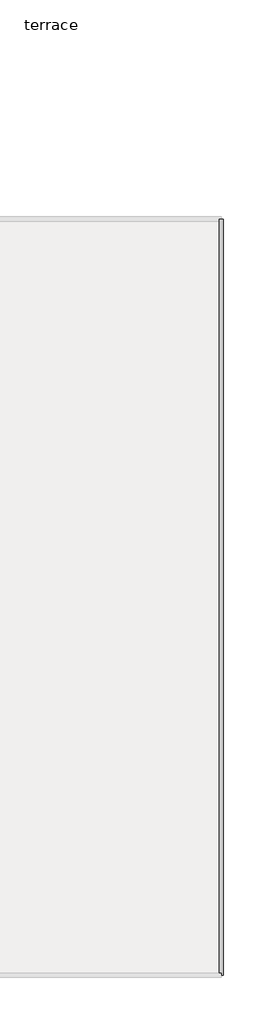
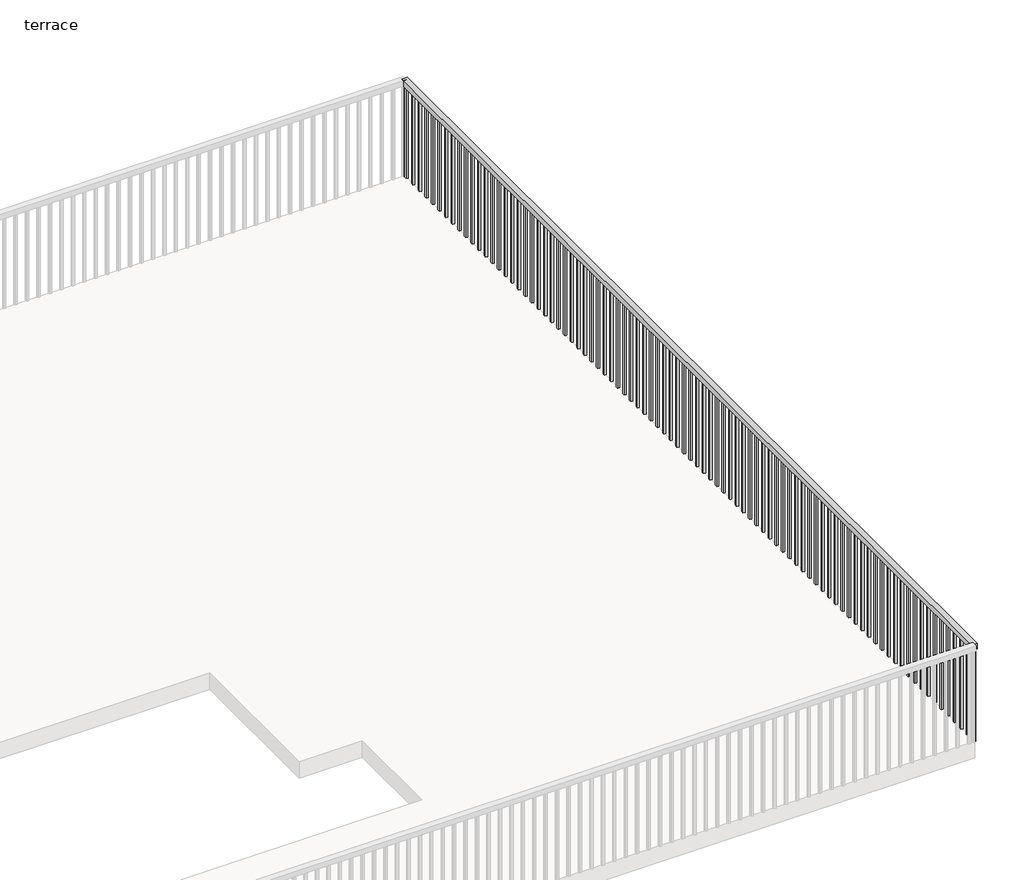
# One storey, part 3 of 4: 1 railing.
"""IFC4 building model written with IfcOpenShell, lengths in millimetres."""

from ifc_helpers import new_model, si_unit, frame, origin, place, context, project, spatial, polyline, outline, extrude, element, save

model = new_model("IFC4")

# Units and contexts
model_context = context("Model", 3, world=origin())
ifc_project = project(units=[si_unit("LENGTHUNIT", "METRE", prefix="MILLI")], contexts=[model_context])

# Site, building, storey
site = spatial("IfcSite", under=ifc_project)
building = spatial("IfcBuilding", under=site)
storey = spatial("IfcBuildingStorey", under=building, Name="terrace", Elevation=7010.4)

# Railing
placement = place(None, origin())
element("IfcRailing", 1, ObjectType="Handrail - Rectangular", at=placement, inside=storey, context=model_context, shape_type="SweptSolid", body=[
    extrude(outline(polyline([(36180.1316163, 5593.0480552), (36129.3316163, 5593.0480552), (36129.3316163, 14362.3980552), (36180.1316163, 14362.3980552), (36180.1316163, 5593.0480552)])), frame((0.0, 0.0, 7874.0), z_axis=(0.0, 0.0, 1.0), x_axis=(1.0, 0.0, 0.0)), (0.0, 0.0, 1.0), 50.8),
    extrude(outline(polyline([(36164.2566163, 14321.1230552), (36145.2066163, 14321.1230552), (36145.2066163, 14340.1730552), (36164.2566163, 14340.1730552), (36164.2566163, 14321.1230552)])), frame((0.0, 0.0, 7010.4), z_axis=(0.0, 0.0, 1.0), x_axis=(1.0, 0.0, 0.0)), (0.0, 0.0, 1.0), 863.6),
    extrude(outline(polyline([(36164.2566163, 14219.5230552), (36145.2066163, 14219.5230552), (36145.2066163, 14238.5730552), (36164.2566163, 14238.5730552), (36164.2566163, 14219.5230552)])), frame((0.0, 0.0, 7010.4), z_axis=(0.0, 0.0, 1.0), x_axis=(1.0, 0.0, 0.0)), (0.0, 0.0, 1.0), 863.6),
    extrude(outline(polyline([(36164.2566163, 14117.9230552), (36145.2066163, 14117.9230552), (36145.2066163, 14136.9730552), (36164.2566163, 14136.9730552), (36164.2566163, 14117.9230552)])), frame((0.0, 0.0, 7010.4), z_axis=(0.0, 0.0, 1.0), x_axis=(1.0, 0.0, 0.0)), (0.0, 0.0, 1.0), 863.6),
    extrude(outline(polyline([(36164.2566163, 14016.3230552), (36145.2066163, 14016.3230552), (36145.2066163, 14035.3730552), (36164.2566163, 14035.3730552), (36164.2566163, 14016.3230552)])), frame((0.0, 0.0, 7010.4), z_axis=(0.0, 0.0, 1.0), x_axis=(1.0, 0.0, 0.0)), (0.0, 0.0, 1.0), 863.6),
    extrude(outline(polyline([(36164.2566163, 13914.7230552), (36145.2066163, 13914.7230552), (36145.2066163, 13933.7730552), (36164.2566163, 13933.7730552), (36164.2566163, 13914.7230552)])), frame((0.0, 0.0, 7010.4), z_axis=(0.0, 0.0, 1.0), x_axis=(1.0, 0.0, 0.0)), (0.0, 0.0, 1.0), 863.6),
    extrude(outline(polyline([(36164.2566163, 13813.1230552), (36145.2066163, 13813.1230552), (36145.2066163, 13832.1730552), (36164.2566163, 13832.1730552), (36164.2566163, 13813.1230552)])), frame((0.0, 0.0, 7010.4), z_axis=(0.0, 0.0, 1.0), x_axis=(1.0, 0.0, 0.0)), (0.0, 0.0, 1.0), 863.6),
    extrude(outline(polyline([(36164.2566163, 13711.5230552), (36145.2066163, 13711.5230552), (36145.2066163, 13730.5730552), (36164.2566163, 13730.5730552), (36164.2566163, 13711.5230552)])), frame((0.0, 0.0, 7010.4), z_axis=(0.0, 0.0, 1.0), x_axis=(1.0, 0.0, 0.0)), (0.0, 0.0, 1.0), 863.6),
    extrude(outline(polyline([(36164.2566163, 13609.9230552), (36145.2066163, 13609.9230552), (36145.2066163, 13628.9730552), (36164.2566163, 13628.9730552), (36164.2566163, 13609.9230552)])), frame((0.0, 0.0, 7010.4), z_axis=(0.0, 0.0, 1.0), x_axis=(1.0, 0.0, 0.0)), (0.0, 0.0, 1.0), 863.6),
    extrude(outline(polyline([(36164.2566163, 13508.3230552), (36145.2066163, 13508.3230552), (36145.2066163, 13527.3730552), (36164.2566163, 13527.3730552), (36164.2566163, 13508.3230552)])), frame((0.0, 0.0, 7010.4), z_axis=(0.0, 0.0, 1.0), x_axis=(1.0, 0.0, 0.0)), (0.0, 0.0, 1.0), 863.6),
    extrude(outline(polyline([(36164.2566163, 13406.7230552), (36145.2066163, 13406.7230552), (36145.2066163, 13425.7730552), (36164.2566163, 13425.7730552), (36164.2566163, 13406.7230552)])), frame((0.0, 0.0, 7010.4), z_axis=(0.0, 0.0, 1.0), x_axis=(1.0, 0.0, 0.0)), (0.0, 0.0, 1.0), 863.6),
    extrude(outline(polyline([(36164.2566163, 13305.1230552), (36145.2066163, 13305.1230552), (36145.2066163, 13324.1730552), (36164.2566163, 13324.1730552), (36164.2566163, 13305.1230552)])), frame((0.0, 0.0, 7010.4), z_axis=(0.0, 0.0, 1.0), x_axis=(1.0, 0.0, 0.0)), (0.0, 0.0, 1.0), 863.6),
    extrude(outline(polyline([(36164.2566163, 13203.5230552), (36145.2066163, 13203.5230552), (36145.2066163, 13222.5730552), (36164.2566163, 13222.5730552), (36164.2566163, 13203.5230552)])), frame((0.0, 0.0, 7010.4), z_axis=(0.0, 0.0, 1.0), x_axis=(1.0, 0.0, 0.0)), (0.0, 0.0, 1.0), 863.6),
    extrude(outline(polyline([(36164.2566163, 13101.9230552), (36145.2066163, 13101.9230552), (36145.2066163, 13120.9730552), (36164.2566163, 13120.9730552), (36164.2566163, 13101.9230552)])), frame((0.0, 0.0, 7010.4), z_axis=(0.0, 0.0, 1.0), x_axis=(1.0, 0.0, 0.0)), (0.0, 0.0, 1.0), 863.6),
    extrude(outline(polyline([(36164.2566163, 13000.3230552), (36145.2066163, 13000.3230552), (36145.2066163, 13019.3730552), (36164.2566163, 13019.3730552), (36164.2566163, 13000.3230552)])), frame((0.0, 0.0, 7010.4), z_axis=(0.0, 0.0, 1.0), x_axis=(1.0, 0.0, 0.0)), (0.0, 0.0, 1.0), 863.6),
    extrude(outline(polyline([(36164.2566163, 12898.7230552), (36145.2066163, 12898.7230552), (36145.2066163, 12917.7730552), (36164.2566163, 12917.7730552), (36164.2566163, 12898.7230552)])), frame((0.0, 0.0, 7010.4), z_axis=(0.0, 0.0, 1.0), x_axis=(1.0, 0.0, 0.0)), (0.0, 0.0, 1.0), 863.6),
    extrude(outline(polyline([(36164.2566163, 12797.1230552), (36145.2066163, 12797.1230552), (36145.2066163, 12816.1730552), (36164.2566163, 12816.1730552), (36164.2566163, 12797.1230552)])), frame((0.0, 0.0, 7010.4), z_axis=(0.0, 0.0, 1.0), x_axis=(1.0, 0.0, 0.0)), (0.0, 0.0, 1.0), 863.6),
    extrude(outline(polyline([(36164.2566163, 12695.5230552), (36145.2066163, 12695.5230552), (36145.2066163, 12714.5730552), (36164.2566163, 12714.5730552), (36164.2566163, 12695.5230552)])), frame((0.0, 0.0, 7010.4), z_axis=(0.0, 0.0, 1.0), x_axis=(1.0, 0.0, 0.0)), (0.0, 0.0, 1.0), 863.6),
    extrude(outline(polyline([(36164.2566163, 12593.9230552), (36145.2066163, 12593.9230552), (36145.2066163, 12612.9730552), (36164.2566163, 12612.9730552), (36164.2566163, 12593.9230552)])), frame((0.0, 0.0, 7010.4), z_axis=(0.0, 0.0, 1.0), x_axis=(1.0, 0.0, 0.0)), (0.0, 0.0, 1.0), 863.6),
    extrude(outline(polyline([(36164.2566163, 12492.3230552), (36145.2066163, 12492.3230552), (36145.2066163, 12511.3730552), (36164.2566163, 12511.3730552), (36164.2566163, 12492.3230552)])), frame((0.0, 0.0, 7010.4), z_axis=(0.0, 0.0, 1.0), x_axis=(1.0, 0.0, 0.0)), (0.0, 0.0, 1.0), 863.6),
    extrude(outline(polyline([(36164.2566163, 12390.7230552), (36145.2066163, 12390.7230552), (36145.2066163, 12409.7730552), (36164.2566163, 12409.7730552), (36164.2566163, 12390.7230552)])), frame((0.0, 0.0, 7010.4), z_axis=(0.0, 0.0, 1.0), x_axis=(1.0, 0.0, 0.0)), (0.0, 0.0, 1.0), 863.6),
    extrude(outline(polyline([(36164.2566163, 12289.1230552), (36145.2066163, 12289.1230552), (36145.2066163, 12308.1730552), (36164.2566163, 12308.1730552), (36164.2566163, 12289.1230552)])), frame((0.0, 0.0, 7010.4), z_axis=(0.0, 0.0, 1.0), x_axis=(1.0, 0.0, 0.0)), (0.0, 0.0, 1.0), 863.6),
    extrude(outline(polyline([(36164.2566163, 12187.5230552), (36145.2066163, 12187.5230552), (36145.2066163, 12206.5730552), (36164.2566163, 12206.5730552), (36164.2566163, 12187.5230552)])), frame((0.0, 0.0, 7010.4), z_axis=(0.0, 0.0, 1.0), x_axis=(1.0, 0.0, 0.0)), (0.0, 0.0, 1.0), 863.6),
    extrude(outline(polyline([(36164.2566163, 12085.9230552), (36145.2066163, 12085.9230552), (36145.2066163, 12104.9730552), (36164.2566163, 12104.9730552), (36164.2566163, 12085.9230552)])), frame((0.0, 0.0, 7010.4), z_axis=(0.0, 0.0, 1.0), x_axis=(1.0, 0.0, 0.0)), (0.0, 0.0, 1.0), 863.6),
    extrude(outline(polyline([(36164.2566163, 11984.3230552), (36145.2066163, 11984.3230552), (36145.2066163, 12003.3730552), (36164.2566163, 12003.3730552), (36164.2566163, 11984.3230552)])), frame((0.0, 0.0, 7010.4), z_axis=(0.0, 0.0, 1.0), x_axis=(1.0, 0.0, 0.0)), (0.0, 0.0, 1.0), 863.6),
    extrude(outline(polyline([(36164.2566163, 11882.7230552), (36145.2066163, 11882.7230552), (36145.2066163, 11901.7730552), (36164.2566163, 11901.7730552), (36164.2566163, 11882.7230552)])), frame((0.0, 0.0, 7010.4), z_axis=(0.0, 0.0, 1.0), x_axis=(1.0, 0.0, 0.0)), (0.0, 0.0, 1.0), 863.6),
    extrude(outline(polyline([(36164.2566163, 11781.1230552), (36145.2066163, 11781.1230552), (36145.2066163, 11800.1730552), (36164.2566163, 11800.1730552), (36164.2566163, 11781.1230552)])), frame((0.0, 0.0, 7010.4), z_axis=(0.0, 0.0, 1.0), x_axis=(1.0, 0.0, 0.0)), (0.0, 0.0, 1.0), 863.6),
    extrude(outline(polyline([(36164.2566163, 11679.5230552), (36145.2066163, 11679.5230552), (36145.2066163, 11698.5730552), (36164.2566163, 11698.5730552), (36164.2566163, 11679.5230552)])), frame((0.0, 0.0, 7010.4), z_axis=(0.0, 0.0, 1.0), x_axis=(1.0, 0.0, 0.0)), (0.0, 0.0, 1.0), 863.6),
    extrude(outline(polyline([(36164.2566163, 11577.9230552), (36145.2066163, 11577.9230552), (36145.2066163, 11596.9730552), (36164.2566163, 11596.9730552), (36164.2566163, 11577.9230552)])), frame((0.0, 0.0, 7010.4), z_axis=(0.0, 0.0, 1.0), x_axis=(1.0, 0.0, 0.0)), (0.0, 0.0, 1.0), 863.6),
    extrude(outline(polyline([(36164.2566163, 11476.3230552), (36145.2066163, 11476.3230552), (36145.2066163, 11495.3730552), (36164.2566163, 11495.3730552), (36164.2566163, 11476.3230552)])), frame((0.0, 0.0, 7010.4), z_axis=(0.0, 0.0, 1.0), x_axis=(1.0, 0.0, 0.0)), (0.0, 0.0, 1.0), 863.6),
    extrude(outline(polyline([(36164.2566163, 11374.7230552), (36145.2066163, 11374.7230552), (36145.2066163, 11393.7730552), (36164.2566163, 11393.7730552), (36164.2566163, 11374.7230552)])), frame((0.0, 0.0, 7010.4), z_axis=(0.0, 0.0, 1.0), x_axis=(1.0, 0.0, 0.0)), (0.0, 0.0, 1.0), 863.6),
    extrude(outline(polyline([(36164.2566163, 11273.1230552), (36145.2066163, 11273.1230552), (36145.2066163, 11292.1730552), (36164.2566163, 11292.1730552), (36164.2566163, 11273.1230552)])), frame((0.0, 0.0, 7010.4), z_axis=(0.0, 0.0, 1.0), x_axis=(1.0, 0.0, 0.0)), (0.0, 0.0, 1.0), 863.6),
    extrude(outline(polyline([(36164.2566163, 11171.5230552), (36145.2066163, 11171.5230552), (36145.2066163, 11190.5730552), (36164.2566163, 11190.5730552), (36164.2566163, 11171.5230552)])), frame((0.0, 0.0, 7010.4), z_axis=(0.0, 0.0, 1.0), x_axis=(1.0, 0.0, 0.0)), (0.0, 0.0, 1.0), 863.6),
    extrude(outline(polyline([(36164.2566163, 11069.9230552), (36145.2066163, 11069.9230552), (36145.2066163, 11088.9730552), (36164.2566163, 11088.9730552), (36164.2566163, 11069.9230552)])), frame((0.0, 0.0, 7010.4), z_axis=(0.0, 0.0, 1.0), x_axis=(1.0, 0.0, 0.0)), (0.0, 0.0, 1.0), 863.6),
    extrude(outline(polyline([(36164.2566163, 10968.3230552), (36145.2066163, 10968.3230552), (36145.2066163, 10987.3730552), (36164.2566163, 10987.3730552), (36164.2566163, 10968.3230552)])), frame((0.0, 0.0, 7010.4), z_axis=(0.0, 0.0, 1.0), x_axis=(1.0, 0.0, 0.0)), (0.0, 0.0, 1.0), 863.6),
    extrude(outline(polyline([(36164.2566163, 10866.7230552), (36145.2066163, 10866.7230552), (36145.2066163, 10885.7730552), (36164.2566163, 10885.7730552), (36164.2566163, 10866.7230552)])), frame((0.0, 0.0, 7010.4), z_axis=(0.0, 0.0, 1.0), x_axis=(1.0, 0.0, 0.0)), (0.0, 0.0, 1.0), 863.6),
    extrude(outline(polyline([(36164.2566163, 10765.1230552), (36145.2066163, 10765.1230552), (36145.2066163, 10784.1730552), (36164.2566163, 10784.1730552), (36164.2566163, 10765.1230552)])), frame((0.0, 0.0, 7010.4), z_axis=(0.0, 0.0, 1.0), x_axis=(1.0, 0.0, 0.0)), (0.0, 0.0, 1.0), 863.6),
    extrude(outline(polyline([(36164.2566163, 10663.5230552), (36145.2066163, 10663.5230552), (36145.2066163, 10682.5730552), (36164.2566163, 10682.5730552), (36164.2566163, 10663.5230552)])), frame((0.0, 0.0, 7010.4), z_axis=(0.0, 0.0, 1.0), x_axis=(1.0, 0.0, 0.0)), (0.0, 0.0, 1.0), 863.6),
    extrude(outline(polyline([(36164.2566163, 10561.9230552), (36145.2066163, 10561.9230552), (36145.2066163, 10580.9730552), (36164.2566163, 10580.9730552), (36164.2566163, 10561.9230552)])), frame((0.0, 0.0, 7010.4), z_axis=(0.0, 0.0, 1.0), x_axis=(1.0, 0.0, 0.0)), (0.0, 0.0, 1.0), 863.6),
    extrude(outline(polyline([(36164.2566163, 10460.3230552), (36145.2066163, 10460.3230552), (36145.2066163, 10479.3730552), (36164.2566163, 10479.3730552), (36164.2566163, 10460.3230552)])), frame((0.0, 0.0, 7010.4), z_axis=(0.0, 0.0, 1.0), x_axis=(1.0, 0.0, 0.0)), (0.0, 0.0, 1.0), 863.6),
    extrude(outline(polyline([(36164.2566163, 10358.7230552), (36145.2066163, 10358.7230552), (36145.2066163, 10377.7730552), (36164.2566163, 10377.7730552), (36164.2566163, 10358.7230552)])), frame((0.0, 0.0, 7010.4), z_axis=(0.0, 0.0, 1.0), x_axis=(1.0, 0.0, 0.0)), (0.0, 0.0, 1.0), 863.6),
    extrude(outline(polyline([(36164.2566163, 10257.1230552), (36145.2066163, 10257.1230552), (36145.2066163, 10276.1730552), (36164.2566163, 10276.1730552), (36164.2566163, 10257.1230552)])), frame((0.0, 0.0, 7010.4), z_axis=(0.0, 0.0, 1.0), x_axis=(1.0, 0.0, 0.0)), (0.0, 0.0, 1.0), 863.6),
    extrude(outline(polyline([(36164.2566163, 10155.5230552), (36145.2066163, 10155.5230552), (36145.2066163, 10174.5730552), (36164.2566163, 10174.5730552), (36164.2566163, 10155.5230552)])), frame((0.0, 0.0, 7010.4), z_axis=(0.0, 0.0, 1.0), x_axis=(1.0, 0.0, 0.0)), (0.0, 0.0, 1.0), 863.6),
    extrude(outline(polyline([(36164.2566163, 10053.9230552), (36145.2066163, 10053.9230552), (36145.2066163, 10072.9730552), (36164.2566163, 10072.9730552), (36164.2566163, 10053.9230552)])), frame((0.0, 0.0, 7010.4), z_axis=(0.0, 0.0, 1.0), x_axis=(1.0, 0.0, 0.0)), (0.0, 0.0, 1.0), 863.6),
    extrude(outline(polyline([(36164.2566163, 9952.3230552), (36145.2066163, 9952.3230552), (36145.2066163, 9971.3730552), (36164.2566163, 9971.3730552), (36164.2566163, 9952.3230552)])), frame((0.0, 0.0, 7010.4), z_axis=(0.0, 0.0, 1.0), x_axis=(1.0, 0.0, 0.0)), (0.0, 0.0, 1.0), 863.6),
    extrude(outline(polyline([(36164.2566163, 9850.7230552), (36145.2066163, 9850.7230552), (36145.2066163, 9869.7730552), (36164.2566163, 9869.7730552), (36164.2566163, 9850.7230552)])), frame((0.0, 0.0, 7010.4), z_axis=(0.0, 0.0, 1.0), x_axis=(1.0, 0.0, 0.0)), (0.0, 0.0, 1.0), 863.6),
    extrude(outline(polyline([(36164.2566163, 9749.1230552), (36145.2066163, 9749.1230552), (36145.2066163, 9768.1730552), (36164.2566163, 9768.1730552), (36164.2566163, 9749.1230552)])), frame((0.0, 0.0, 7010.4), z_axis=(0.0, 0.0, 1.0), x_axis=(1.0, 0.0, 0.0)), (0.0, 0.0, 1.0), 863.6),
    extrude(outline(polyline([(36164.2566163, 9647.5230552), (36145.2066163, 9647.5230552), (36145.2066163, 9666.5730552), (36164.2566163, 9666.5730552), (36164.2566163, 9647.5230552)])), frame((0.0, 0.0, 7010.4), z_axis=(0.0, 0.0, 1.0), x_axis=(1.0, 0.0, 0.0)), (0.0, 0.0, 1.0), 863.6),
    extrude(outline(polyline([(36164.2566163, 9545.9230552), (36145.2066163, 9545.9230552), (36145.2066163, 9564.9730552), (36164.2566163, 9564.9730552), (36164.2566163, 9545.9230552)])), frame((0.0, 0.0, 7010.4), z_axis=(0.0, 0.0, 1.0), x_axis=(1.0, 0.0, 0.0)), (0.0, 0.0, 1.0), 863.6),
    extrude(outline(polyline([(36164.2566163, 9444.3230552), (36145.2066163, 9444.3230552), (36145.2066163, 9463.3730552), (36164.2566163, 9463.3730552), (36164.2566163, 9444.3230552)])), frame((0.0, 0.0, 7010.4), z_axis=(0.0, 0.0, 1.0), x_axis=(1.0, 0.0, 0.0)), (0.0, 0.0, 1.0), 863.6),
    extrude(outline(polyline([(36164.2566163, 9342.7230552), (36145.2066163, 9342.7230552), (36145.2066163, 9361.7730552), (36164.2566163, 9361.7730552), (36164.2566163, 9342.7230552)])), frame((0.0, 0.0, 7010.4), z_axis=(0.0, 0.0, 1.0), x_axis=(1.0, 0.0, 0.0)), (0.0, 0.0, 1.0), 863.6),
    extrude(outline(polyline([(36164.2566163, 9241.1230552), (36145.2066163, 9241.1230552), (36145.2066163, 9260.1730552), (36164.2566163, 9260.1730552), (36164.2566163, 9241.1230552)])), frame((0.0, 0.0, 7010.4), z_axis=(0.0, 0.0, 1.0), x_axis=(1.0, 0.0, 0.0)), (0.0, 0.0, 1.0), 863.6),
    extrude(outline(polyline([(36164.2566163, 9139.5230552), (36145.2066163, 9139.5230552), (36145.2066163, 9158.5730552), (36164.2566163, 9158.5730552), (36164.2566163, 9139.5230552)])), frame((0.0, 0.0, 7010.4), z_axis=(0.0, 0.0, 1.0), x_axis=(1.0, 0.0, 0.0)), (0.0, 0.0, 1.0), 863.6),
    extrude(outline(polyline([(36164.2566163, 9037.9230552), (36145.2066163, 9037.9230552), (36145.2066163, 9056.9730552), (36164.2566163, 9056.9730552), (36164.2566163, 9037.9230552)])), frame((0.0, 0.0, 7010.4), z_axis=(0.0, 0.0, 1.0), x_axis=(1.0, 0.0, 0.0)), (0.0, 0.0, 1.0), 863.6),
    extrude(outline(polyline([(36164.2566163, 8936.3230552), (36145.2066163, 8936.3230552), (36145.2066163, 8955.3730552), (36164.2566163, 8955.3730552), (36164.2566163, 8936.3230552)])), frame((0.0, 0.0, 7010.4), z_axis=(0.0, 0.0, 1.0), x_axis=(1.0, 0.0, 0.0)), (0.0, 0.0, 1.0), 863.6),
    extrude(outline(polyline([(36164.2566163, 8834.7230552), (36145.2066163, 8834.7230552), (36145.2066163, 8853.7730552), (36164.2566163, 8853.7730552), (36164.2566163, 8834.7230552)])), frame((0.0, 0.0, 7010.4), z_axis=(0.0, 0.0, 1.0), x_axis=(1.0, 0.0, 0.0)), (0.0, 0.0, 1.0), 863.6),
    extrude(outline(polyline([(36164.2566163, 8733.1230552), (36145.2066163, 8733.1230552), (36145.2066163, 8752.1730552), (36164.2566163, 8752.1730552), (36164.2566163, 8733.1230552)])), frame((0.0, 0.0, 7010.4), z_axis=(0.0, 0.0, 1.0), x_axis=(1.0, 0.0, 0.0)), (0.0, 0.0, 1.0), 863.6),
    extrude(outline(polyline([(36164.2566163, 8631.5230552), (36145.2066163, 8631.5230552), (36145.2066163, 8650.5730552), (36164.2566163, 8650.5730552), (36164.2566163, 8631.5230552)])), frame((0.0, 0.0, 7010.4), z_axis=(0.0, 0.0, 1.0), x_axis=(1.0, 0.0, 0.0)), (0.0, 0.0, 1.0), 863.6),
    extrude(outline(polyline([(36164.2566163, 8529.9230552), (36145.2066163, 8529.9230552), (36145.2066163, 8548.9730552), (36164.2566163, 8548.9730552), (36164.2566163, 8529.9230552)])), frame((0.0, 0.0, 7010.4), z_axis=(0.0, 0.0, 1.0), x_axis=(1.0, 0.0, 0.0)), (0.0, 0.0, 1.0), 863.6),
    extrude(outline(polyline([(36164.2566163, 8428.3230552), (36145.2066163, 8428.3230552), (36145.2066163, 8447.3730552), (36164.2566163, 8447.3730552), (36164.2566163, 8428.3230552)])), frame((0.0, 0.0, 7010.4), z_axis=(0.0, 0.0, 1.0), x_axis=(1.0, 0.0, 0.0)), (0.0, 0.0, 1.0), 863.6),
    extrude(outline(polyline([(36164.2566163, 8326.7230552), (36145.2066163, 8326.7230552), (36145.2066163, 8345.7730552), (36164.2566163, 8345.7730552), (36164.2566163, 8326.7230552)])), frame((0.0, 0.0, 7010.4), z_axis=(0.0, 0.0, 1.0), x_axis=(1.0, 0.0, 0.0)), (0.0, 0.0, 1.0), 863.6),
    extrude(outline(polyline([(36164.2566163, 8225.1230552), (36145.2066163, 8225.1230552), (36145.2066163, 8244.1730552), (36164.2566163, 8244.1730552), (36164.2566163, 8225.1230552)])), frame((0.0, 0.0, 7010.4), z_axis=(0.0, 0.0, 1.0), x_axis=(1.0, 0.0, 0.0)), (0.0, 0.0, 1.0), 863.6),
    extrude(outline(polyline([(36164.2566163, 8123.5230552), (36145.2066163, 8123.5230552), (36145.2066163, 8142.5730552), (36164.2566163, 8142.5730552), (36164.2566163, 8123.5230552)])), frame((0.0, 0.0, 7010.4), z_axis=(0.0, 0.0, 1.0), x_axis=(1.0, 0.0, 0.0)), (0.0, 0.0, 1.0), 863.6),
    extrude(outline(polyline([(36164.2566163, 8021.9230552), (36145.2066163, 8021.9230552), (36145.2066163, 8040.9730552), (36164.2566163, 8040.9730552), (36164.2566163, 8021.9230552)])), frame((0.0, 0.0, 7010.4), z_axis=(0.0, 0.0, 1.0), x_axis=(1.0, 0.0, 0.0)), (0.0, 0.0, 1.0), 863.6),
    extrude(outline(polyline([(36164.2566163, 7920.3230552), (36145.2066163, 7920.3230552), (36145.2066163, 7939.3730552), (36164.2566163, 7939.3730552), (36164.2566163, 7920.3230552)])), frame((0.0, 0.0, 7010.4), z_axis=(0.0, 0.0, 1.0), x_axis=(1.0, 0.0, 0.0)), (0.0, 0.0, 1.0), 863.6),
    extrude(outline(polyline([(36164.2566163, 7818.7230552), (36145.2066163, 7818.7230552), (36145.2066163, 7837.7730552), (36164.2566163, 7837.7730552), (36164.2566163, 7818.7230552)])), frame((0.0, 0.0, 7010.4), z_axis=(0.0, 0.0, 1.0), x_axis=(1.0, 0.0, 0.0)), (0.0, 0.0, 1.0), 863.6),
    extrude(outline(polyline([(36164.2566163, 7717.1230552), (36145.2066163, 7717.1230552), (36145.2066163, 7736.1730552), (36164.2566163, 7736.1730552), (36164.2566163, 7717.1230552)])), frame((0.0, 0.0, 7010.4), z_axis=(0.0, 0.0, 1.0), x_axis=(1.0, 0.0, 0.0)), (0.0, 0.0, 1.0), 863.6),
    extrude(outline(polyline([(36164.2566163, 7615.5230552), (36145.2066163, 7615.5230552), (36145.2066163, 7634.5730552), (36164.2566163, 7634.5730552), (36164.2566163, 7615.5230552)])), frame((0.0, 0.0, 7010.4), z_axis=(0.0, 0.0, 1.0), x_axis=(1.0, 0.0, 0.0)), (0.0, 0.0, 1.0), 863.6),
    extrude(outline(polyline([(36164.2566163, 7513.9230552), (36145.2066163, 7513.9230552), (36145.2066163, 7532.9730552), (36164.2566163, 7532.9730552), (36164.2566163, 7513.9230552)])), frame((0.0, 0.0, 7010.4), z_axis=(0.0, 0.0, 1.0), x_axis=(1.0, 0.0, 0.0)), (0.0, 0.0, 1.0), 863.6),
    extrude(outline(polyline([(36164.2566163, 7412.3230552), (36145.2066163, 7412.3230552), (36145.2066163, 7431.3730552), (36164.2566163, 7431.3730552), (36164.2566163, 7412.3230552)])), frame((0.0, 0.0, 7010.4), z_axis=(0.0, 0.0, 1.0), x_axis=(1.0, 0.0, 0.0)), (0.0, 0.0, 1.0), 863.6),
    extrude(outline(polyline([(36164.2566163, 7310.7230552), (36145.2066163, 7310.7230552), (36145.2066163, 7329.7730552), (36164.2566163, 7329.7730552), (36164.2566163, 7310.7230552)])), frame((0.0, 0.0, 7010.4), z_axis=(0.0, 0.0, 1.0), x_axis=(1.0, 0.0, 0.0)), (0.0, 0.0, 1.0), 863.6),
    extrude(outline(polyline([(36164.2566163, 7209.1230552), (36145.2066163, 7209.1230552), (36145.2066163, 7228.1730552), (36164.2566163, 7228.1730552), (36164.2566163, 7209.1230552)])), frame((0.0, 0.0, 7010.4), z_axis=(0.0, 0.0, 1.0), x_axis=(1.0, 0.0, 0.0)), (0.0, 0.0, 1.0), 863.6),
    extrude(outline(polyline([(36164.2566163, 7107.5230552), (36145.2066163, 7107.5230552), (36145.2066163, 7126.5730552), (36164.2566163, 7126.5730552), (36164.2566163, 7107.5230552)])), frame((0.0, 0.0, 7010.4), z_axis=(0.0, 0.0, 1.0), x_axis=(1.0, 0.0, 0.0)), (0.0, 0.0, 1.0), 863.6),
    extrude(outline(polyline([(36164.2566163, 7005.9230552), (36145.2066163, 7005.9230552), (36145.2066163, 7024.9730552), (36164.2566163, 7024.9730552), (36164.2566163, 7005.9230552)])), frame((0.0, 0.0, 7010.4), z_axis=(0.0, 0.0, 1.0), x_axis=(1.0, 0.0, 0.0)), (0.0, 0.0, 1.0), 863.6),
    extrude(outline(polyline([(36164.2566163, 6904.3230552), (36145.2066163, 6904.3230552), (36145.2066163, 6923.3730552), (36164.2566163, 6923.3730552), (36164.2566163, 6904.3230552)])), frame((0.0, 0.0, 7010.4), z_axis=(0.0, 0.0, 1.0), x_axis=(1.0, 0.0, 0.0)), (0.0, 0.0, 1.0), 863.6),
    extrude(outline(polyline([(36164.2566163, 6802.7230552), (36145.2066163, 6802.7230552), (36145.2066163, 6821.7730552), (36164.2566163, 6821.7730552), (36164.2566163, 6802.7230552)])), frame((0.0, 0.0, 7010.4), z_axis=(0.0, 0.0, 1.0), x_axis=(1.0, 0.0, 0.0)), (0.0, 0.0, 1.0), 863.6),
    extrude(outline(polyline([(36164.2566163, 6701.1230552), (36145.2066163, 6701.1230552), (36145.2066163, 6720.1730552), (36164.2566163, 6720.1730552), (36164.2566163, 6701.1230552)])), frame((0.0, 0.0, 7010.4), z_axis=(0.0, 0.0, 1.0), x_axis=(1.0, 0.0, 0.0)), (0.0, 0.0, 1.0), 863.6),
    extrude(outline(polyline([(36164.2566163, 6599.5230552), (36145.2066163, 6599.5230552), (36145.2066163, 6618.5730552), (36164.2566163, 6618.5730552), (36164.2566163, 6599.5230552)])), frame((0.0, 0.0, 7010.4), z_axis=(0.0, 0.0, 1.0), x_axis=(1.0, 0.0, 0.0)), (0.0, 0.0, 1.0), 863.6),
    extrude(outline(polyline([(36164.2566163, 6497.9230552), (36145.2066163, 6497.9230552), (36145.2066163, 6516.9730552), (36164.2566163, 6516.9730552), (36164.2566163, 6497.9230552)])), frame((0.0, 0.0, 7010.4), z_axis=(0.0, 0.0, 1.0), x_axis=(1.0, 0.0, 0.0)), (0.0, 0.0, 1.0), 863.6),
    extrude(outline(polyline([(36164.2566163, 6396.3230552), (36145.2066163, 6396.3230552), (36145.2066163, 6415.3730552), (36164.2566163, 6415.3730552), (36164.2566163, 6396.3230552)])), frame((0.0, 0.0, 7010.4), z_axis=(0.0, 0.0, 1.0), x_axis=(1.0, 0.0, 0.0)), (0.0, 0.0, 1.0), 863.6),
    extrude(outline(polyline([(36164.2566163, 6294.7230552), (36145.2066163, 6294.7230552), (36145.2066163, 6313.7730552), (36164.2566163, 6313.7730552), (36164.2566163, 6294.7230552)])), frame((0.0, 0.0, 7010.4), z_axis=(0.0, 0.0, 1.0), x_axis=(1.0, 0.0, 0.0)), (0.0, 0.0, 1.0), 863.6),
    extrude(outline(polyline([(36164.2566163, 6193.1230552), (36145.2066163, 6193.1230552), (36145.2066163, 6212.1730552), (36164.2566163, 6212.1730552), (36164.2566163, 6193.1230552)])), frame((0.0, 0.0, 7010.4), z_axis=(0.0, 0.0, 1.0), x_axis=(1.0, 0.0, 0.0)), (0.0, 0.0, 1.0), 863.6),
    extrude(outline(polyline([(36164.2566163, 6091.5230552), (36145.2066163, 6091.5230552), (36145.2066163, 6110.5730552), (36164.2566163, 6110.5730552), (36164.2566163, 6091.5230552)])), frame((0.0, 0.0, 7010.4), z_axis=(0.0, 0.0, 1.0), x_axis=(1.0, 0.0, 0.0)), (0.0, 0.0, 1.0), 863.6),
    extrude(outline(polyline([(36164.2566163, 5989.9230552), (36145.2066163, 5989.9230552), (36145.2066163, 6008.9730552), (36164.2566163, 6008.9730552), (36164.2566163, 5989.9230552)])), frame((0.0, 0.0, 7010.4), z_axis=(0.0, 0.0, 1.0), x_axis=(1.0, 0.0, 0.0)), (0.0, 0.0, 1.0), 863.6),
    extrude(outline(polyline([(36164.2566163, 5888.3230552), (36145.2066163, 5888.3230552), (36145.2066163, 5907.3730552), (36164.2566163, 5907.3730552), (36164.2566163, 5888.3230552)])), frame((0.0, 0.0, 7010.4), z_axis=(0.0, 0.0, 1.0), x_axis=(1.0, 0.0, 0.0)), (0.0, 0.0, 1.0), 863.6),
    extrude(outline(polyline([(36164.2566163, 5786.7230552), (36145.2066163, 5786.7230552), (36145.2066163, 5805.7730552), (36164.2566163, 5805.7730552), (36164.2566163, 5786.7230552)])), frame((0.0, 0.0, 7010.4), z_axis=(0.0, 0.0, 1.0), x_axis=(1.0, 0.0, 0.0)), (0.0, 0.0, 1.0), 863.6),
    extrude(outline(polyline([(36164.2566163, 5685.1230552), (36145.2066163, 5685.1230552), (36145.2066163, 5704.1730552), (36164.2566163, 5704.1730552), (36164.2566163, 5685.1230552)])), frame((0.0, 0.0, 7010.4), z_axis=(0.0, 0.0, 1.0), x_axis=(1.0, 0.0, 0.0)), (0.0, 0.0, 1.0), 863.6),
    extrude(outline(polyline([(36164.2566163, 14343.3480552), (36145.2066163, 14343.3480552), (36145.2066163, 14362.3980552), (36164.2566163, 14362.3980552), (36164.2566163, 14343.3480552)])), frame((0.0, 0.0, 7010.4), z_axis=(0.0, 0.0, 1.0), x_axis=(1.0, 0.0, 0.0)), (0.0, 0.0, 1.0), 863.6),
    extrude(outline(polyline([(36164.2566163, 5593.0480552), (36145.2066163, 5593.0480552), (36145.2066163, 5612.0980552), (36164.2566163, 5612.0980552), (36164.2566163, 5593.0480552)])), frame((0.0, 0.0, 7010.4), z_axis=(0.0, 0.0, 1.0), x_axis=(1.0, 0.0, 0.0)), (0.0, 0.0, 1.0), 863.6),
])

save(model, "model.ifc")

# Revit data of these elements
# Type "Handrail - Rectangular"
#   Assembly Code = "C2010400"
#   built-in parameter 1008612 = 0.0416667 (stored number, unit not read)
#   built-in parameter 1008611 = 0.0416667 (stored number, unit not read)
#   built-in parameter 1008609 = 0.333333 (stored number, unit not read)
#   built-in parameter 1008604 = 0.166667 (stored number, unit not read)
#   built-in parameter 1008603 = 0.166667 (stored number, unit not read)
#   Railing Height = 3' - 0"
#   built-in parameter 1008630 = 2
#   built-in parameter 1008610 = 2
#   built-in parameter 1008618 = Baluster - Square : 3/4"
# Element 1 (IfcRailing, "Handrail - Rectangular")
#   Phase Created = New Construction
